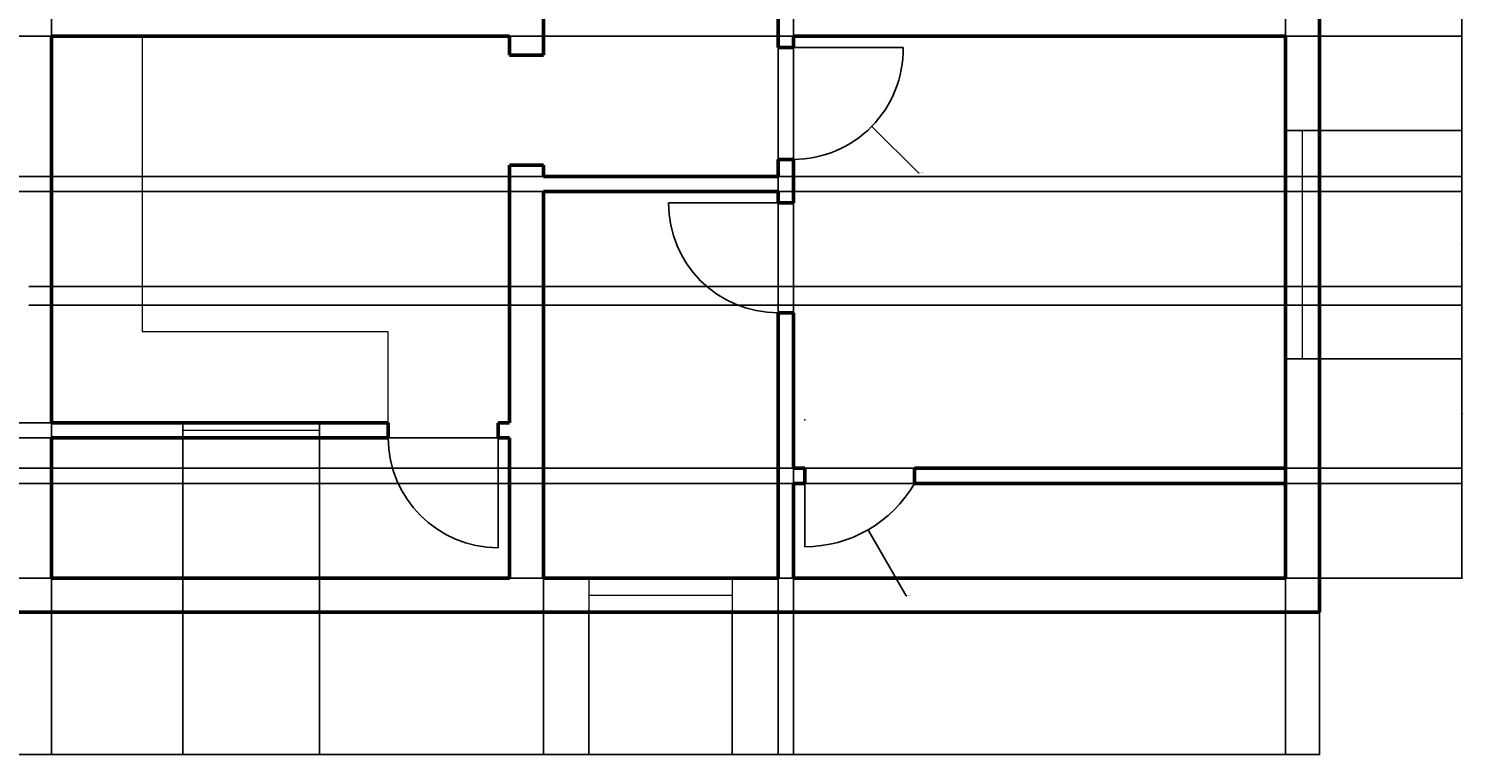
# Model space of a CAD drawing. Units: inches. Extents: x 2479 to 3284, y 2154 to 2936.
# Tile 5 of 8: x 2905 to 3284, y 2154 to 2346. Entities that reach past the tile are written whole.
import ezdxf

# ---------------------------------------------------------------- set-up
doc = ezdxf.new("R2010")
doc.units = ezdxf.units.IN
for name, color, linetype, lineweight in [('A-ANNO-DIMS', 2, 'Continuous', 18), ('A-DOOR', 3, 'Continuous', 25), ('A-FLOR-CASE', 8, 'Continuous', 18), ('A-GLAZ', 4, 'Continuous', 18), ('A-WALL', 7, 'Continuous', 50)]:
    doc.layers.add(name, color=color, linetype=linetype, lineweight=lineweight)
doc.styles.get("Standard").update_dxf_attribs({"font": 'arial.ttf'})
doc.dimstyles.get("Standard").update_dxf_attribs({"dimtxt": 0.18, "dimasz": 0.18, "dimexe": 0.18, "dimexo": 0.0625, "dimgap": 0.09, "dimtad": 0, "dimtih": 1, "dimtoh": 1, "dimdec": 4, "dimzin": 0, "dimdsep": 46, "dimtxsty": 'Standard', "dimcen": 0.09, "dimadec": 0, "dimazin": 0, "dimtfac": 1, "dimtdec": 4, "dimtofl": 0, "dimtmove": 0, "dimatfit": 3, "dimfxl": 1, "dimtolj": 1, "dimtzin": 0, "dimarcsym": 0})

# ---------------------------------------------------------------- blocks, each defined once
blk = doc.blocks.new('DOOR-SWING-29IN')
blk.add_line((29, 0), (0, 0))
blk.add_arc((29, 0), 29, 90, 180)
blk = doc.blocks.new('*D7')
at = {"layer": 'A-ANNO-DIMS', "color": 0, "lineweight": -2, "transparency": 16777216}
for p, q in [((2517.21, 2191.68), (2517.21, 2153.96)), ((3246.21, 2191.68), (3246.21, 2153.96)), ((2517.39, 2154.14), (2881.42, 2154.14)), ((3246.03, 2154.14), (2882, 2154.14))]:
    blk.add_line(p, q, dxfattribs=at)
at = {"layer": 'A-ANNO-DIMS', "color": 0, "transparency": 16777216}
for points in [[(2517.39, 2154.17), (2517.39, 2154.11), (2517.21, 2154.14)], [(3246.03, 2154.17), (3246.03, 2154.11), (3246.21, 2154.14)]]:
    blk.add_solid(points, dxfattribs=at)
at = {"layer": 'Defpoints', "color": 0, "transparency": 16777216}
for p in [(2517.21, 2191.74), (3246.21, 2191.74), (3246.21, 2154.14)]:
    blk.add_point(p, dxfattribs=at)
at = {"layer": 'A-ANNO-DIMS', "color": 0, "transparency": 16777216, "insert": (2881.71, 2154.14), "char_height": 0.18, "attachment_point": 5}
blk.add_mtext('\\A1;729', dxfattribs=at)
blk = doc.blocks.new('*D13')
at = {"layer": 'A-ANNO-DIMS', "color": 0, "lineweight": -2, "transparency": 16777216}
for p, q in [((2905.27, 2272.74), (3283.99, 2272.74)), ((3283.81, 2272.56), (3283.81, 2236.92)), ((3283.81, 2200.92), (3283.81, 2236.56)), ((2905.27, 2200.74), (3283.99, 2200.74))]:
    blk.add_line(p, q, dxfattribs=at)
at = {"layer": 'A-ANNO-DIMS', "color": 0, "transparency": 16777216}
for points in [[(3283.78, 2272.56), (3283.84, 2272.56), (3283.81, 2272.74)], [(3283.78, 2200.92), (3283.84, 2200.92), (3283.81, 2200.74)]]:
    blk.add_solid(points, dxfattribs=at)
at = {"layer": 'Defpoints', "color": 0, "transparency": 16777216}
for p in [(2905.21, 2272.74), (3283.81, 2272.74), (2905.21, 2200.74)]:
    blk.add_point(p, dxfattribs=at)
at = {"layer": 'A-ANNO-DIMS', "color": 0, "transparency": 16777216, "insert": (3283.81, 2236.74), "char_height": 0.18, "attachment_point": 5}
blk.add_mtext('\\A1;72', dxfattribs=at)
blk = doc.blocks.new('*D14')
at = {"layer": 'A-ANNO-DIMS', "color": 0, "lineweight": -2, "transparency": 16777216}
for p, q in [((2905.27, 2277.74), (3283.99, 2277.74)), ((3283.81, 2277.56), (3283.81, 2275.42)), ((3283.81, 2272.92), (3283.81, 2275.06)), ((2905.27, 2272.74), (3283.99, 2272.74))]:
    blk.add_line(p, q, dxfattribs=at)
at = {"layer": 'A-ANNO-DIMS', "color": 0, "transparency": 16777216}
for points in [[(3283.78, 2277.56), (3283.84, 2277.56), (3283.81, 2277.74)], [(3283.78, 2272.92), (3283.84, 2272.92), (3283.81, 2272.74)]]:
    blk.add_solid(points, dxfattribs=at)
at = {"layer": 'Defpoints', "color": 0, "transparency": 16777216}
for p in [(2905.21, 2277.74), (3283.81, 2277.74), (2905.21, 2272.74)]:
    blk.add_point(p, dxfattribs=at)
at = {"layer": 'A-ANNO-DIMS', "color": 0, "transparency": 16777216, "insert": (3283.81, 2275.24), "char_height": 0.18, "attachment_point": 5}
blk.add_mtext('\\A1;5', dxfattribs=at)
blk = doc.blocks.new('*D17')
at = {"layer": 'A-ANNO-DIMS', "color": 0, "lineweight": -2, "transparency": 16777216}
for p, q in [((2905.27, 2350.74), (3283.99, 2350.74)), ((3283.81, 2350.56), (3283.81, 2314.42)), ((3283.81, 2277.92), (3283.81, 2314.06)), ((2905.27, 2277.74), (3283.99, 2277.74))]:
    blk.add_line(p, q, dxfattribs=at)
at = {"layer": 'A-ANNO-DIMS', "color": 0, "transparency": 16777216}
for points in [[(3283.78, 2350.56), (3283.84, 2350.56), (3283.81, 2350.74)], [(3283.78, 2277.92), (3283.84, 2277.92), (3283.81, 2277.74)]]:
    blk.add_solid(points, dxfattribs=at)
at = {"layer": 'Defpoints', "color": 0, "transparency": 16777216}
for p in [(2905.21, 2350.74), (3283.81, 2350.74), (2905.21, 2277.74)]:
    blk.add_point(p, dxfattribs=at)
at = {"layer": 'A-ANNO-DIMS', "color": 0, "transparency": 16777216, "insert": (3283.81, 2314.24), "char_height": 0.18, "attachment_point": 5}
blk.add_mtext('\\A1;73', dxfattribs=at)
blk = doc.blocks.new('*D87')
at = {"layer": 'A-ANNO-DIMS', "color": 0, "lineweight": -2, "transparency": 16777216}
for p, q in [((2911.21, 2542.68), (2911.21, 2153.96)), ((3103.21, 2542.68), (3103.21, 2153.96)), ((2911.39, 2154.14), (3006.93, 2154.14)), ((3103.03, 2154.14), (3007.49, 2154.14))]:
    blk.add_line(p, q, dxfattribs=at)
at = {"layer": 'A-ANNO-DIMS', "color": 0, "transparency": 16777216}
for points in [[(2911.39, 2154.17), (2911.39, 2154.11), (2911.21, 2154.14)], [(3103.03, 2154.17), (3103.03, 2154.11), (3103.21, 2154.14)]]:
    blk.add_solid(points, dxfattribs=at)
at = {"layer": 'Defpoints', "color": 0, "transparency": 16777216}
for p in [(2911.21, 2542.74), (3103.21, 2542.74), (3103.21, 2154.14)]:
    blk.add_point(p, dxfattribs=at)
at = {"layer": 'A-ANNO-DIMS', "color": 0, "transparency": 16777216, "insert": (3007.21, 2154.14), "char_height": 0.18, "attachment_point": 5}
blk.add_mtext('\\A1;192', dxfattribs=at)
blk = doc.blocks.new('*D88')
at = {"layer": 'A-ANNO-DIMS', "color": 0, "lineweight": -2, "transparency": 16777216}
for p, q in [((3107.21, 2542.68), (3107.21, 2153.96)), ((3237.21, 2542.68), (3237.21, 2153.96)), ((3107.39, 2154.14), (3171.93, 2154.14)), ((3237.03, 2154.14), (3172.49, 2154.14))]:
    blk.add_line(p, q, dxfattribs=at)
at = {"layer": 'A-ANNO-DIMS', "color": 0, "transparency": 16777216}
for points in [[(3107.39, 2154.17), (3107.39, 2154.11), (3107.21, 2154.14)], [(3237.03, 2154.17), (3237.03, 2154.11), (3237.21, 2154.14)]]:
    blk.add_solid(points, dxfattribs=at)
at = {"layer": 'Defpoints', "color": 0, "transparency": 16777216}
for p in [(3107.21, 2542.74), (3237.21, 2542.74), (3237.21, 2154.14)]:
    blk.add_point(p, dxfattribs=at)
at = {"layer": 'A-ANNO-DIMS', "color": 0, "transparency": 16777216, "insert": (3172.21, 2154.14), "char_height": 0.18, "attachment_point": 5}
blk.add_mtext('\\A1;130', dxfattribs=at)
blk = doc.blocks.new('*D106')
at = {"layer": 'A-ANNO-DIMS', "color": 0, "lineweight": -2, "transparency": 16777216}
for p, q in [((2727.27, 2225.74), (3283.99, 2225.74)), ((3283.81, 2225.56), (3283.81, 2213.42)), ((3283.81, 2200.92), (3283.81, 2213.06)), ((2839.27, 2200.74), (3283.99, 2200.74))]:
    blk.add_line(p, q, dxfattribs=at)
at = {"layer": 'A-ANNO-DIMS', "color": 0, "transparency": 16777216}
for points in [[(3283.78, 2225.56), (3283.84, 2225.56), (3283.81, 2225.74)], [(3283.78, 2200.92), (3283.84, 2200.92), (3283.81, 2200.74)]]:
    blk.add_solid(points, dxfattribs=at)
at = {"layer": 'Defpoints', "color": 0, "transparency": 16777216}
for p in [(2727.21, 2225.74), (3283.81, 2225.74), (2839.21, 2200.74)]:
    blk.add_point(p, dxfattribs=at)
at = {"layer": 'A-ANNO-DIMS', "color": 0, "transparency": 16777216, "insert": (3283.81, 2213.24), "char_height": 0.18, "attachment_point": 5}
blk.add_mtext('\\A1;25', dxfattribs=at)
blk = doc.blocks.new('*D107')
at = {"layer": 'A-ANNO-DIMS', "color": 0, "lineweight": -2, "transparency": 16777216}
for p, q in [((2721.27, 2302.74), (3283.99, 2302.74)), ((3283.81, 2302.56), (3283.81, 2266.42)), ((3283.81, 2229.92), (3283.81, 2266.06)), ((2839.27, 2229.74), (3283.99, 2229.74))]:
    blk.add_line(p, q, dxfattribs=at)
at = {"layer": 'A-ANNO-DIMS', "color": 0, "transparency": 16777216}
for points in [[(3283.78, 2302.56), (3283.84, 2302.56), (3283.81, 2302.74)], [(3283.78, 2229.92), (3283.84, 2229.92), (3283.81, 2229.74)]]:
    blk.add_solid(points, dxfattribs=at)
at = {"layer": 'Defpoints', "color": 0, "transparency": 16777216}
for p in [(2721.21, 2302.74), (2839.21, 2229.74), (3283.81, 2229.74)]:
    blk.add_point(p, dxfattribs=at)
at = {"layer": 'A-ANNO-DIMS', "color": 0, "transparency": 16777216, "insert": (3283.81, 2266.24), "char_height": 0.18, "attachment_point": 5}
blk.add_mtext('\\A1;73', dxfattribs=at)
blk = doc.blocks.new('*D108')
at = {"layer": 'A-ANNO-DIMS', "color": 0, "lineweight": -2, "transparency": 16777216}
for p, q in [((2839.27, 2343.74), (3283.99, 2343.74)), ((3283.81, 2343.56), (3283.81, 2325.42)), ((3283.81, 2306.92), (3283.81, 2325.06)), ((2721.27, 2306.74), (3283.99, 2306.74))]:
    blk.add_line(p, q, dxfattribs=at)
at = {"layer": 'A-ANNO-DIMS', "color": 0, "transparency": 16777216}
for points in [[(3283.78, 2343.56), (3283.84, 2343.56), (3283.81, 2343.74)], [(3283.78, 2306.92), (3283.84, 2306.92), (3283.81, 2306.74)]]:
    blk.add_solid(points, dxfattribs=at)
at = {"layer": 'Defpoints', "color": 0, "transparency": 16777216}
for p in [(2839.21, 2343.74), (3283.81, 2343.74), (2721.21, 2306.74)]:
    blk.add_point(p, dxfattribs=at)
at = {"layer": 'A-ANNO-DIMS', "color": 0, "transparency": 16777216, "insert": (3283.81, 2325.24), "char_height": 0.18, "attachment_point": 5}
blk.add_mtext('\\A1;37', dxfattribs=at)
blk = doc.blocks.new('*D112')
at = {"layer": 'A-ANNO-DIMS', "color": 0, "lineweight": -2, "transparency": 16777216}
for p, q in [((2945.91, 2241.68), (2945.91, 2153.96)), ((2982.05, 2241.68), (2982.05, 2153.96)), ((2946.09, 2154.14), (2963.59, 2154.14)), ((2981.87, 2154.14), (2964.37, 2154.14))]:
    blk.add_line(p, q, dxfattribs=at)
at = {"layer": 'A-ANNO-DIMS', "color": 0, "transparency": 16777216}
for points in [[(2946.09, 2154.17), (2946.09, 2154.11), (2945.91, 2154.14)], [(2981.87, 2154.17), (2981.87, 2154.11), (2982.05, 2154.14)]]:
    blk.add_solid(points, dxfattribs=at)
at = {"layer": 'Defpoints', "color": 0, "transparency": 16777216}
for p in [(2945.91, 2241.74), (2982.05, 2241.74), (2982.05, 2154.14)]:
    blk.add_point(p, dxfattribs=at)
at = {"layer": 'A-ANNO-DIMS', "color": 0, "transparency": 16777216, "insert": (2963.98, 2154.14), "char_height": 0.18, "attachment_point": 5}
blk.add_mtext('\\A1;36.14', dxfattribs=at)
blk = doc.blocks.new('*D113')
at = {"layer": 'A-ANNO-DIMS', "color": 0, "lineweight": -2, "transparency": 16777216}
for p, q in [((2911.21, 2241.68), (2911.21, 2153.96)), ((2945.91, 2241.68), (2945.91, 2153.96)), ((2911.39, 2154.14), (2928.24, 2154.14)), ((2945.73, 2154.14), (2928.88, 2154.14))]:
    blk.add_line(p, q, dxfattribs=at)
at = {"layer": 'A-ANNO-DIMS', "color": 0, "transparency": 16777216}
for points in [[(2911.39, 2154.17), (2911.39, 2154.11), (2911.21, 2154.14)], [(2945.73, 2154.17), (2945.73, 2154.11), (2945.91, 2154.14)]]:
    blk.add_solid(points, dxfattribs=at)
at = {"layer": 'Defpoints', "color": 0, "transparency": 16777216}
for p in [(2911.21, 2241.74), (2945.91, 2241.74), (2945.91, 2154.14)]:
    blk.add_point(p, dxfattribs=at)
at = {"layer": 'A-ANNO-DIMS', "color": 0, "transparency": 16777216, "insert": (2928.56, 2154.14), "char_height": 0.18, "attachment_point": 5}
blk.add_mtext('\\A1;34.7', dxfattribs=at)
blk = doc.blocks.new('*D114')
at = {"layer": 'A-ANNO-DIMS', "color": 0, "lineweight": -2, "transparency": 16777216}
for p, q in [((3041.21, 2200.68), (3041.21, 2153.96)), ((3053.15, 2191.68), (3053.15, 2153.96)), ((3041.39, 2154.14), (3046.73, 2154.14)), ((3052.97, 2154.14), (3047.64, 2154.14))]:
    blk.add_line(p, q, dxfattribs=at)
at = {"layer": 'A-ANNO-DIMS', "color": 0, "transparency": 16777216}
for points in [[(3041.39, 2154.17), (3041.39, 2154.11), (3041.21, 2154.14)], [(3052.97, 2154.17), (3052.97, 2154.11), (3053.15, 2154.14)]]:
    blk.add_solid(points, dxfattribs=at)
at = {"layer": 'Defpoints', "color": 0, "transparency": 16777216}
for p in [(3041.21, 2200.74), (3053.15, 2191.74), (3053.15, 2154.14)]:
    blk.add_point(p, dxfattribs=at)
at = {"layer": 'A-ANNO-DIMS', "color": 0, "transparency": 16777216, "insert": (3047.18, 2154.14), "char_height": 0.18, "attachment_point": 5}
blk.add_mtext('\\A1;11.945', dxfattribs=at)
blk = doc.blocks.new('*D115')
at = {"layer": 'A-ANNO-DIMS', "color": 0, "lineweight": -2, "transparency": 16777216}
for p, q in [((3053.15, 2191.68), (3053.15, 2153.96)), ((3091.08, 2191.68), (3091.08, 2153.96)), ((3053.33, 2154.14), (3071.72, 2154.14)), ((3090.9, 2154.14), (3072.51, 2154.14))]:
    blk.add_line(p, q, dxfattribs=at)
at = {"layer": 'A-ANNO-DIMS', "color": 0, "transparency": 16777216}
for points in [[(3053.33, 2154.17), (3053.33, 2154.11), (3053.15, 2154.14)], [(3090.9, 2154.17), (3090.9, 2154.11), (3091.08, 2154.14)]]:
    blk.add_solid(points, dxfattribs=at)
at = {"layer": 'Defpoints', "color": 0, "transparency": 16777216}
for p in [(3053.15, 2191.74), (3091.08, 2191.74), (3091.08, 2154.14)]:
    blk.add_point(p, dxfattribs=at)
at = {"layer": 'A-ANNO-DIMS', "color": 0, "transparency": 16777216, "insert": (3072.12, 2154.14), "char_height": 0.18, "attachment_point": 5}
blk.add_mtext('\\A1;37.93', dxfattribs=at)
blk = doc.blocks.new('*D116')
at = {"layer": 'A-ANNO-DIMS', "color": 0, "lineweight": -2, "transparency": 16777216}
for p, q in [((3103.21, 2200.68), (3103.21, 2153.96)), ((3091.08, 2191.68), (3091.08, 2153.96)), ((3091.26, 2154.14), (3096.69, 2154.14)), ((3103.03, 2154.14), (3097.6, 2154.14))]:
    blk.add_line(p, q, dxfattribs=at)
at = {"layer": 'A-ANNO-DIMS', "color": 0, "transparency": 16777216}
for points in [[(3091.26, 2154.17), (3091.26, 2154.11), (3091.08, 2154.14)], [(3103.03, 2154.17), (3103.03, 2154.11), (3103.21, 2154.14)]]:
    blk.add_solid(points, dxfattribs=at)
at = {"layer": 'Defpoints', "color": 0, "transparency": 16777216}
for p in [(3103.21, 2200.74), (3091.08, 2191.74), (3103.21, 2154.14)]:
    blk.add_point(p, dxfattribs=at)
at = {"layer": 'A-ANNO-DIMS', "color": 0, "transparency": 16777216, "insert": (3097.14, 2154.14), "char_height": 0.18, "attachment_point": 5}
blk.add_mtext('\\A1;12.128', dxfattribs=at)
blk = doc.blocks.new('*D117')
at = {"layer": 'A-ANNO-DIMS', "color": 0, "lineweight": -2, "transparency": 16777216}
for p, q in [((3107.21, 2200.68), (3107.21, 2153.96)), ((3237.21, 2200.68), (3237.21, 2153.96)), ((3107.39, 2154.14), (3171.93, 2154.14)), ((3237.03, 2154.14), (3172.49, 2154.14))]:
    blk.add_line(p, q, dxfattribs=at)
at = {"layer": 'A-ANNO-DIMS', "color": 0, "transparency": 16777216}
for points in [[(3107.39, 2154.17), (3107.39, 2154.11), (3107.21, 2154.14)], [(3237.03, 2154.17), (3237.03, 2154.11), (3237.21, 2154.14)]]:
    blk.add_solid(points, dxfattribs=at)
at = {"layer": 'Defpoints', "color": 0, "transparency": 16777216}
for p in [(3107.21, 2200.74), (3237.21, 2200.74), (3237.21, 2154.14)]:
    blk.add_point(p, dxfattribs=at)
at = {"layer": 'A-ANNO-DIMS', "color": 0, "transparency": 16777216, "insert": (3172.21, 2154.14), "char_height": 0.18, "attachment_point": 5}
blk.add_mtext('\\A1;130', dxfattribs=at)
blk = doc.blocks.new('*D118')
at = {"layer": 'A-ANNO-DIMS', "color": 0, "lineweight": -2, "transparency": 16777216}
for p, q in [((3237.27, 2225.74), (3283.99, 2225.74)), ((3283.81, 2225.56), (3283.81, 2213.42)), ((3283.81, 2200.92), (3283.81, 2213.06)), ((3237.27, 2200.74), (3283.99, 2200.74))]:
    blk.add_line(p, q, dxfattribs=at)
at = {"layer": 'A-ANNO-DIMS', "color": 0, "transparency": 16777216}
for points in [[(3283.78, 2225.56), (3283.84, 2225.56), (3283.81, 2225.74)], [(3283.78, 2200.92), (3283.84, 2200.92), (3283.81, 2200.74)]]:
    blk.add_solid(points, dxfattribs=at)
at = {"layer": 'Defpoints', "color": 0, "transparency": 16777216}
for p in [(3237.21, 2225.74), (3283.81, 2225.74), (3237.21, 2200.74)]:
    blk.add_point(p, dxfattribs=at)
at = {"layer": 'A-ANNO-DIMS', "color": 0, "transparency": 16777216, "insert": (3283.81, 2213.24), "char_height": 0.18, "attachment_point": 5}
blk.add_mtext('\\A1;25', dxfattribs=at)
blk = doc.blocks.new('*D119')
at = {"layer": 'A-ANNO-DIMS', "color": 0, "lineweight": -2, "transparency": 16777216}
for p, q in [((3237.27, 2258.57), (3283.99, 2258.57)), ((3283.81, 2258.39), (3283.81, 2244.34)), ((3283.81, 2229.92), (3283.81, 2243.97)), ((3237.27, 2229.74), (3283.99, 2229.74))]:
    blk.add_line(p, q, dxfattribs=at)
at = {"layer": 'A-ANNO-DIMS', "color": 0, "transparency": 16777216}
for points in [[(3283.78, 2258.39), (3283.84, 2258.39), (3283.81, 2258.57)], [(3283.78, 2229.92), (3283.84, 2229.92), (3283.81, 2229.74)]]:
    blk.add_solid(points, dxfattribs=at)
at = {"layer": 'Defpoints', "color": 0, "transparency": 16777216}
for p in [(3237.21, 2258.57), (3283.81, 2258.57), (3237.21, 2229.74)]:
    blk.add_point(p, dxfattribs=at)
at = {"layer": 'A-ANNO-DIMS', "color": 0, "transparency": 16777216, "insert": (3283.81, 2244.16), "char_height": 0.18, "attachment_point": 5}
blk.add_mtext('\\A1;28.834', dxfattribs=at)
blk = doc.blocks.new('*D120')
at = {"layer": 'A-ANNO-DIMS', "color": 0, "lineweight": -2, "transparency": 16777216}
for p, q in [((3237.27, 2318.9), (3283.99, 2318.9)), ((3283.81, 2318.72), (3283.81, 2288.92)), ((3283.81, 2258.75), (3283.81, 2288.55)), ((3237.27, 2258.57), (3283.99, 2258.57))]:
    blk.add_line(p, q, dxfattribs=at)
at = {"layer": 'A-ANNO-DIMS', "color": 0, "transparency": 16777216}
for points in [[(3283.78, 2318.72), (3283.84, 2318.72), (3283.81, 2318.9)], [(3283.78, 2258.75), (3283.84, 2258.75), (3283.81, 2258.57)]]:
    blk.add_solid(points, dxfattribs=at)
at = {"layer": 'Defpoints', "color": 0, "transparency": 16777216}
for p in [(3237.21, 2318.9), (3283.81, 2318.9), (3237.21, 2258.57)]:
    blk.add_point(p, dxfattribs=at)
at = {"layer": 'A-ANNO-DIMS', "color": 0, "transparency": 16777216, "insert": (3283.81, 2288.74), "char_height": 0.18, "attachment_point": 5}
blk.add_mtext('\\A1;60.33', dxfattribs=at)
blk = doc.blocks.new('*D121')
at = {"layer": 'A-ANNO-DIMS', "color": 0, "lineweight": -2, "transparency": 16777216}
for p, q in [((3237.27, 2343.74), (3283.99, 2343.74)), ((3283.81, 2343.56), (3283.81, 2331.5)), ((3283.81, 2319.08), (3283.81, 2331.14)), ((3237.27, 2318.9), (3283.99, 2318.9))]:
    blk.add_line(p, q, dxfattribs=at)
at = {"layer": 'A-ANNO-DIMS', "color": 0, "transparency": 16777216}
for points in [[(3283.78, 2343.56), (3283.84, 2343.56), (3283.81, 2343.74)], [(3283.78, 2319.08), (3283.84, 2319.08), (3283.81, 2318.9)]]:
    blk.add_solid(points, dxfattribs=at)
at = {"layer": 'Defpoints', "color": 0, "transparency": 16777216}
for p in [(3237.21, 2343.74), (3283.81, 2343.74), (3237.21, 2318.9)]:
    blk.add_point(p, dxfattribs=at)
at = {"layer": 'A-ANNO-DIMS', "color": 0, "transparency": 16777216, "insert": (3283.81, 2331.32), "char_height": 0.18, "attachment_point": 5}
blk.add_mtext('\\A1;24.84', dxfattribs=at)
blk = doc.blocks.new('*D128')
at = {"layer": 'A-ANNO-DIMS', "color": 0, "lineweight": -2, "transparency": 16777216}
for p, q in [((3032.15, 2237.74), (2479.43, 2237.74)), ((2479.61, 2237.56), (2479.61, 2219.42)), ((2479.61, 2200.92), (2479.61, 2219.06)), ((3032.15, 2200.74), (2479.43, 2200.74))]:
    blk.add_line(p, q, dxfattribs=at)
at = {"layer": 'A-ANNO-DIMS', "color": 0, "transparency": 16777216}
for points in [[(2479.58, 2237.56), (2479.64, 2237.56), (2479.61, 2237.74)], [(2479.58, 2200.92), (2479.64, 2200.92), (2479.61, 2200.74)]]:
    blk.add_solid(points, dxfattribs=at)
at = {"layer": 'Defpoints', "color": 0, "transparency": 16777216}
for p in [(2479.61, 2237.74), (3032.21, 2237.74), (3032.21, 2200.74)]:
    blk.add_point(p, dxfattribs=at)
at = {"layer": 'A-ANNO-DIMS', "color": 0, "transparency": 16777216, "insert": (2479.61, 2219.24), "char_height": 0.18, "attachment_point": 5}
blk.add_mtext('\\A1;37', dxfattribs=at)
blk = doc.blocks.new('*D129')
at = {"layer": 'A-ANNO-DIMS', "color": 0, "lineweight": -2, "transparency": 16777216}
for p, q in [((3041.15, 2302.74), (2479.43, 2302.74)), ((2479.61, 2302.56), (2479.61, 2272.42)), ((2479.61, 2241.92), (2479.61, 2272.06)), ((2911.15, 2241.74), (2479.43, 2241.74))]:
    blk.add_line(p, q, dxfattribs=at)
at = {"layer": 'A-ANNO-DIMS', "color": 0, "transparency": 16777216}
for points in [[(2479.58, 2302.56), (2479.64, 2302.56), (2479.61, 2302.74)], [(2479.58, 2241.92), (2479.64, 2241.92), (2479.61, 2241.74)]]:
    blk.add_solid(points, dxfattribs=at)
at = {"layer": 'Defpoints', "color": 0, "transparency": 16777216}
for p in [(2479.61, 2302.74), (3041.21, 2302.74), (2911.21, 2241.74)]:
    blk.add_point(p, dxfattribs=at)
at = {"layer": 'A-ANNO-DIMS', "color": 0, "transparency": 16777216, "insert": (2479.61, 2272.24), "char_height": 0.18, "attachment_point": 5}
blk.add_mtext('\\A1;61', dxfattribs=at)
blk = doc.blocks.new('*D130')
at = {"layer": 'A-ANNO-DIMS', "color": 0, "lineweight": -2, "transparency": 16777216}
for p, q in [((2911.15, 2343.74), (2479.43, 2343.74)), ((2479.61, 2343.56), (2479.61, 2325.42)), ((2479.61, 2306.92), (2479.61, 2325.06)), ((3041.15, 2306.74), (2479.43, 2306.74))]:
    blk.add_line(p, q, dxfattribs=at)
at = {"layer": 'A-ANNO-DIMS', "color": 0, "transparency": 16777216}
for points in [[(2479.58, 2343.56), (2479.64, 2343.56), (2479.61, 2343.74)], [(2479.58, 2306.92), (2479.64, 2306.92), (2479.61, 2306.74)]]:
    blk.add_solid(points, dxfattribs=at)
at = {"layer": 'Defpoints', "color": 0, "transparency": 16777216}
for p in [(2479.61, 2343.74), (2911.21, 2343.74), (3041.21, 2306.74)]:
    blk.add_point(p, dxfattribs=at)
at = {"layer": 'A-ANNO-DIMS', "color": 0, "transparency": 16777216, "insert": (2479.61, 2325.24), "char_height": 0.18, "attachment_point": 5}
blk.add_mtext('\\A1;37', dxfattribs=at)
blk = doc.blocks.new('*D135')
at = {"layer": 'A-ANNO-DIMS', "color": 0, "lineweight": -2, "transparency": 16777216}
for p, q in [((3110.12, 2242.5), (3110.3, 2242.5)), ((3110.21, 2242.41), (3110.21, 2242.59)), ((3136.99, 2196.08), (3127.04, 2213.33)), ((3137.17, 2196.08), (3136.99, 2196.08))]:
    blk.add_line(p, q, dxfattribs=at)
at = {"layer": 'A-ANNO-DIMS', "color": 0, "transparency": 16777216}
blk.add_solid([(3127.07, 2213.35), (3127.01, 2213.32), (3126.95, 2213.49)], dxfattribs=at)
at = {"layer": 'Defpoints', "color": 0, "transparency": 16777216}
for p in [(3110.21, 2242.5), (3126.95, 2213.49)]:
    blk.add_point(p, dxfattribs=at)
at = {"layer": 'A-ANNO-DIMS', "color": 0, "transparency": 16777216, "insert": (3137.72, 2196.08), "char_height": 0.18, "attachment_point": 5}
blk.add_mtext('\\A1;R33.496', dxfattribs=at)
blk = doc.blocks.new('*D138')
at = {"layer": 'A-ANNO-DIMS', "color": 0, "lineweight": -2, "transparency": 16777216}
for p, q in [((3107.12, 2340.26), (3107.3, 2340.26)), ((3107.21, 2340.17), (3107.21, 2340.35)), ((3140.29, 2307.72), (3128.01, 2319.8)), ((3140.47, 2307.72), (3140.29, 2307.72))]:
    blk.add_line(p, q, dxfattribs=at)
at = {"layer": 'A-ANNO-DIMS', "color": 0, "transparency": 16777216}
blk.add_solid([(3128.03, 2319.82), (3127.99, 2319.78), (3127.89, 2319.92)], dxfattribs=at)
at = {"layer": 'Defpoints', "color": 0, "transparency": 16777216}
for p in [(3107.21, 2340.26), (3127.89, 2319.92)]:
    blk.add_point(p, dxfattribs=at)
at = {"layer": 'A-ANNO-DIMS', "color": 0, "transparency": 16777216, "insert": (3141.02, 2307.72), "char_height": 0.18, "attachment_point": 5}
blk.add_mtext('\\A1;R29.004', dxfattribs=at)

msp = doc.modelspace()

# ---------------------------------------------------------------- linework, layer by layer
at = {"layer": 'A-DOOR'}
for p, q in [((3107.2088, 2340.7397), (3136.2088, 2340.7397)), ((3110.2088, 2225.7397), (3110.2088, 2209.0063))]:
    msp.add_line(p, q, dxfattribs=at)
for centre, radius, end in [((3107.2088, 2340.263), 29.0039, 0.941762), ((3110.2088, 2242.5024), 33.496, 329.971194)]:
    msp.add_arc(centre, radius, 270, end, dxfattribs=at)
at = {"layer": 'A-FLOR-CASE'}
for p, q in [((2935.2088, 2343.7397), (2935.2088, 2265.7397)), ((3000.2088, 2265.7397), (2935.2088, 2265.7397)), ((3000.2088, 2241.7397), (3000.2088, 2265.7397))]:
    msp.add_line(p, q, dxfattribs=at)
at = {"layer": 'A-GLAZ'}
for p, q in [((3237.2088, 2318.8992), (3246.2088, 2318.8992)), ((3241.7088, 2258.5738), (3241.7088, 2318.8992)), ((3237.2088, 2258.5738), (3246.2088, 2258.5738)), ((2945.9107, 2241.7397), (2945.9107, 2237.7397)), ((2982.0487, 2241.7397), (2982.0487, 2237.7397)), ((2945.9107, 2239.7397), (2982.0487, 2239.7397)), ((3053.1536, 2200.7397), (3053.1536, 2191.7397)), ((3091.0807, 2200.7397), (3091.0807, 2191.7397)), ((3053.1536, 2196.2397), (3091.0807, 2196.2397))]:
    msp.add_line(p, q, dxfattribs=at)
at = {"layer": 'A-WALL'}
for p, q in [((3246.2088, 2191.7397), (3246.2088, 2897.7397)), ((3103.2088, 2403.7397), (3103.2088, 2340.7397)), ((3041.2088, 2354.1045), (3041.2088, 2338.7702)), ((3032.2088, 2343.7397), (2911.2088, 2343.7397)), ((2911.2088, 2343.7397), (2911.2088, 2241.7397)), ((3032.2088, 2343.7397), (3032.2088, 2338.7702)), ((3237.2088, 2343.7397), (3107.2088, 2343.7397)), ((3107.2088, 2343.7397), (3107.2088, 2340.7397)), ((3237.2088, 2200.7397), (3237.2088, 2343.7397)), ((3041.2088, 2338.7702), (3032.2088, 2338.7702)), ((3107.2088, 2340.7397), (3103.2088, 2340.7397)), ((3041.2088, 2309.7397), (3032.2088, 2309.7397)), ((3032.2088, 2309.7397), (3032.2088, 2241.7397)), ((3041.2088, 2309.7397), (3041.2088, 2306.7397)), ((3107.2088, 2311.2591), (3103.2088, 2311.2591)), ((3103.2088, 2311.2591), (3103.2088, 2306.7397)), ((3107.2088, 2311.2591), (3107.2088, 2299.7397)), ((3041.2088, 2306.7397), (3103.2088, 2306.7397)), ((3041.2088, 2302.7397), (3103.2088, 2302.7397)), ((3041.2088, 2302.7397), (3041.2088, 2200.7397)), ((3103.2088, 2302.7397), (3103.2088, 2299.7397)), ((3103.2088, 2299.7397), (3107.2088, 2299.7397)), ((3103.2088, 2270.7397), (3107.2088, 2270.7397)), ((3103.2088, 2270.7397), (3103.2088, 2200.7397)), ((3107.2088, 2270.7397), (3107.2088, 2229.7397)), ((3000.2088, 2241.7397), (2911.2088, 2241.7397)), ((3000.2088, 2241.7397), (3000.2088, 2237.7397)), ((3032.2088, 2241.7397), (3029.2088, 2241.7397)), ((3029.2088, 2241.7397), (3029.2088, 2237.7397)), ((3000.2088, 2237.7397), (2911.2088, 2237.7397)), ((2911.2088, 2237.7397), (2911.2088, 2200.7397)), ((3032.2088, 2237.7397), (3029.2088, 2237.7397)), ((3032.2088, 2237.7397), (3032.2088, 2200.7397)), ((3110.2088, 2229.7397), (3107.2088, 2229.7397)), ((3110.2088, 2229.7397), (3110.2088, 2225.7397)), ((3237.2088, 2229.7397), (3139.2088, 2229.7397)), ((3139.2088, 2229.7397), (3139.2088, 2225.7397)), ((3110.2088, 2225.7397), (3107.2088, 2225.7397)), ((3107.2088, 2225.7397), (3107.2088, 2200.7397)), ((3237.2088, 2225.7397), (3139.2088, 2225.7397)), ((2911.2088, 2200.7397), (3032.2088, 2200.7397)), ((3041.2088, 2200.7397), (3103.2088, 2200.7397)), ((3107.2088, 2200.7397), (3237.2088, 2200.7397)), ((2517.2088, 2191.7397), (3246.2088, 2191.7397))]:
    msp.add_line(p, q, dxfattribs=at)

# ---------------------------------------------------------------- block references
at = {"layer": 'A-DOOR', "extrusion": (0, 0, -1), "zscale": -1, "rotation": 180}
msp.add_blockref('DOOR-SWING-29IN', (-3074.2088, 2299.7397), dxfattribs=at)
at = {"layer": 'A-DOOR', "rotation": 90}
msp.add_blockref('DOOR-SWING-29IN', (3029.2088, 2208.7397), dxfattribs=at)

# ---------------------------------------------------------------- dimensions: what is measured, and where the dimension line sits
at = {"layer": 'A-ANNO-DIMS'}
for base, p1, p2, override, picture, middle in [((3103.2088, 2154.1397), (2911.2088, 2542.7397), (3103.2088, 2542.7397), {"dimdec": 0, "dimlfac": 1, "dimrnd": 0, "dimzin": 0, "dimdsep": 46, "dimlunit": 2}, '*D87', (3007.2088, 2154.1397)), ((3237.2088, 2154.1397), (3107.2088, 2542.7397), (3237.2088, 2542.7397), {"dimdec": 0, "dimlfac": 1, "dimrnd": 0, "dimzin": 0, "dimdsep": 46, "dimlunit": 2}, '*D88', (3172.2088, 2154.1397)), ((2945.9107, 2154.1397), (2911.2088, 2241.7397), (2945.9107, 2241.7397), {"dimdec": 1, "dimlfac": 1, "dimrnd": 0, "dimzin": 0, "dimdsep": 46, "dimlunit": 2}, '*D113', (2928.5597, 2154.1397)), ((2982.0487, 2154.1397), (2945.9107, 2241.7397), (2982.0487, 2241.7397), {"dimdec": 2, "dimlfac": 1, "dimrnd": 0, "dimzin": 0, "dimdsep": 46, "dimlunit": 2}, '*D112', (2963.9797, 2154.1397)), ((3053.1536, 2154.1397), (3041.2088, 2200.7397), (3053.1536, 2191.7397), {"dimdec": 3, "dimlfac": 1, "dimrnd": 0, "dimzin": 0, "dimdsep": 46, "dimlunit": 2}, '*D114', (3047.1812, 2154.1397)), ((3103.2088, 2154.1397), (3091.0807, 2191.7397), (3103.2088, 2200.7397), {"dimdec": 3, "dimlfac": 1, "dimrnd": 0, "dimzin": 0, "dimdsep": 46, "dimlunit": 2}, '*D116', (3097.1448, 2154.1397)), ((3237.2088, 2154.1397), (3107.2088, 2200.7397), (3237.2088, 2200.7397), {"dimdec": 0, "dimlfac": 1, "dimrnd": 0, "dimzin": 0, "dimdsep": 46, "dimlunit": 2}, '*D117', (3172.2088, 2154.1397)), ((3246.2088, 2154.1397), (2517.2088, 2191.7397), (3246.2088, 2191.7397), {"dimdec": 0, "dimlfac": 1, "dimrnd": 0, "dimzin": 0, "dimdsep": 46, "dimlunit": 2}, '*D7', (2881.7088, 2154.1397)), ((3091.0807, 2154.1397), (3053.1536, 2191.7397), (3091.0807, 2191.7397), {"dimdec": 2, "dimlfac": 1, "dimrnd": 0, "dimzin": 0, "dimdsep": 46, "dimlunit": 2}, '*D115', (3072.1171, 2154.1397))]:
    dim = msp.add_linear_dim(base=base, p1=p1, p2=p2, dimstyle='Standard', override=override, dxfattribs=at)
    dim.commit()
    dim.dimension.update_dxf_attribs({"geometry": picture, "text_midpoint": middle})
for base, p1, p2, override, picture, middle in [((3283.8088, 2350.7397), (2905.2088, 2277.7397), (2905.2088, 2350.7397), {"dimdec": 0, "dimlfac": 1, "dimrnd": 0, "dimzin": 0, "dimdsep": 46, "dimlunit": 2}, '*D17', (3283.8088, 2314.2397)), ((2479.6088, 2343.7397), (3041.2088, 2306.7397), (2911.2088, 2343.7397), {"dimdec": 0, "dimlfac": 1, "dimrnd": 0, "dimzin": 0, "dimdsep": 46, "dimlunit": 2}, '*D130', (2479.6088, 2325.2397)), ((3283.8088, 2343.7397), (2721.2088, 2306.7397), (2839.2088, 2343.7397), {"dimdec": 0, "dimlfac": 1, "dimrnd": 0, "dimzin": 0, "dimdsep": 46, "dimlunit": 2}, '*D108', (3283.8088, 2325.2397)), ((3283.8088, 2343.7397), (3237.2088, 2318.8992), (3237.2088, 2343.7397), {"dimdec": 2, "dimlfac": 1, "dimrnd": 0, "dimzin": 0, "dimdsep": 46, "dimlunit": 2}, '*D121', (3283.8088, 2331.3195)), ((3283.8088, 2318.8992), (3237.2088, 2258.5738), (3237.2088, 2318.8992), {"dimdec": 2, "dimlfac": 1, "dimrnd": 0, "dimzin": 0, "dimdsep": 46, "dimlunit": 2}, '*D120', (3283.8088, 2288.7365)), ((2479.6088, 2302.7397), (2911.2088, 2241.7397), (3041.2088, 2302.7397), {"dimdec": 0, "dimlfac": 1, "dimrnd": 0, "dimzin": 0, "dimdsep": 46, "dimlunit": 2}, '*D129', (2479.6088, 2272.2397)), ((3283.8088, 2229.7397), (2721.2088, 2302.7397), (2839.2088, 2229.7397), {"dimdec": 0, "dimlfac": 1, "dimrnd": 0, "dimzin": 0, "dimdsep": 46, "dimlunit": 2}, '*D107', (3283.8088, 2266.2397)), ((3283.8088, 2277.7397), (2905.2088, 2272.7397), (2905.2088, 2277.7397), {"dimdec": 0, "dimlfac": 1, "dimrnd": 0, "dimzin": 0, "dimdsep": 46, "dimlunit": 2}, '*D14', (3283.8088, 2275.2397)), ((3283.8088, 2272.7397), (2905.2088, 2200.7397), (2905.2088, 2272.7397), {"dimdec": 0, "dimlfac": 1, "dimrnd": 0, "dimzin": 0, "dimdsep": 46, "dimlunit": 2}, '*D13', (3283.8088, 2236.7397)), ((3283.8088, 2258.5738), (3237.2088, 2229.7397), (3237.2088, 2258.5738), {"dimdec": 3, "dimlfac": 1, "dimrnd": 0, "dimzin": 0, "dimdsep": 46, "dimlunit": 2}, '*D119', (3283.8088, 2244.1568)), ((2479.6088, 2237.7397), (3032.2088, 2200.7397), (3032.2088, 2237.7397), {"dimdec": 0, "dimlfac": 1, "dimrnd": 0, "dimzin": 0, "dimdsep": 46, "dimlunit": 2}, '*D128', (2479.6088, 2219.2397)), ((3283.8088, 2225.7397), (2839.2088, 2200.7397), (2727.2088, 2225.7397), {"dimdec": 0, "dimlfac": 1, "dimrnd": 0, "dimzin": 0, "dimdsep": 46, "dimlunit": 2}, '*D106', (3283.8088, 2213.2397)), ((3283.8088, 2225.7397), (3237.2088, 2200.7397), (3237.2088, 2225.7397), {"dimdec": 0, "dimlfac": 1, "dimrnd": 0, "dimzin": 0, "dimdsep": 46, "dimlunit": 2}, '*D118', (3283.8088, 2213.2397))]:
    dim = msp.add_linear_dim(base=base, p1=p1, p2=p2, angle=90, dimstyle='Standard', override=override, dxfattribs=at)
    dim.commit()
    dim.dimension.update_dxf_attribs({"geometry": picture, "text_midpoint": middle})
for center, mpoint, picture, middle in [((3107.2088, 2340.263), (3127.8856, 2319.9234), '*D138', (3141.021, 2307.7197)), ((3110.2088, 2242.5024), (3126.95, 2213.49), '*D135', (3137.7244, 2196.0826))]:
    dim = msp.add_radius_dim(center=center, mpoint=mpoint, dimstyle='Standard', override={"dimdec": 3, "dimlfac": 1, "dimrnd": 0, "dimzin": 0, "dimdsep": 46, "dimlunit": 2}, dxfattribs=at)
    dim.commit()
    dim.dimension.update_dxf_attribs({"geometry": picture, "text_midpoint": middle, "dimtype": 164})

doc.saveas('drawing.dxf')
